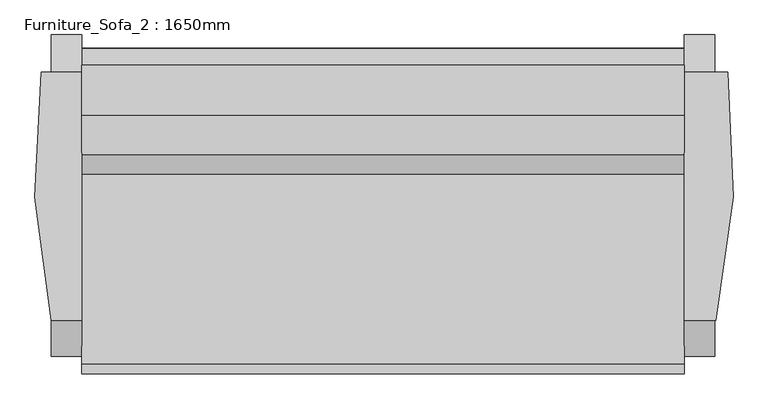
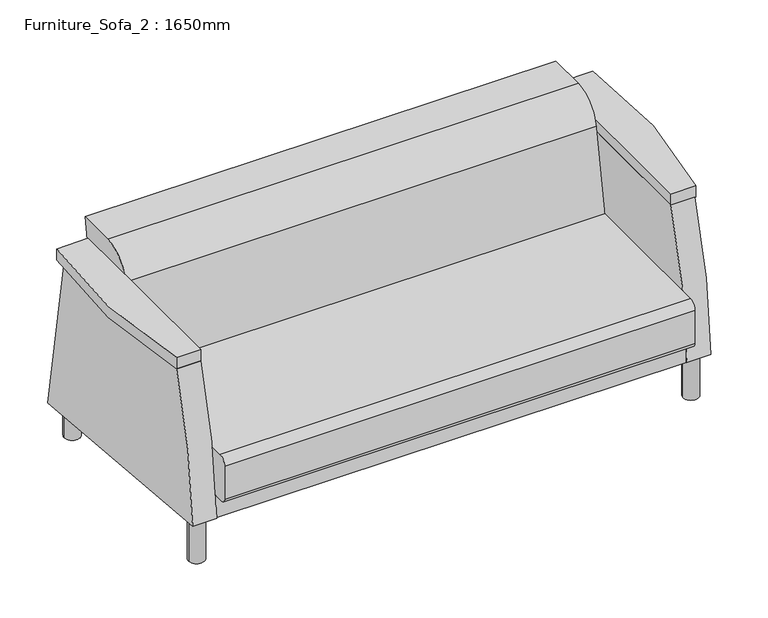
"""IFC4 building model written with IfcOpenShell, lengths in millimetres: furniture geometry, Furniture_Sofa_2 : 1650mm."""

from ifc_helpers import new_model, si_unit, point, frame, frame_2d, origin, origin_with_axes, place, context, project, spatial, polyline, circle_curve, trimmed, segment, composite_curve, outline, extrude, source, transform, mapped, element, save


def furniture_sofa_2_1650mm_c7211d0d(model_context):
    return source(origin(), model_context, "Body", "SweptSolid", [
        extrude(outline(composite_curve([segment(trimmed(circle_curve(frame_2d((-116.5901639, 351.2509954)), 25.4), [point((-141.9901639, 351.2509954))], [point((-116.5901639, 376.6509954))], False, "CARTESIAN"), True, "CONTINUOUS"), segment(polyline([(-116.5901639, 376.6509954), (355.3895541, 376.6509954), (402.1988177, 642.1195211)]), True, "CONTINUOUS"), segment(trimmed(circle_curve(frame_2d((502.2552854, 624.4768662)), 101.6), [point((402.1988177, 642.1195211))], [point((502.2552854, 726.0768662))], False, "CARTESIAN"), True, "CONTINUOUS"), segment(polyline([(502.2552854, 726.0768662), (626.3344485, 726.0768662), (609.5377828, 620.1719187), (667.6541767, 224.2509954), (-126.1151639, 224.2509954)]), True, "CONTINUOUS"), segment(trimmed(circle_curve(frame_2d((-126.1151639, 240.1259954)), 15.875), [point((-126.1151639, 224.2509954))], [point((-141.9901639, 240.1259954))], False, "CARTESIAN"), True, "CONTINUOUS"), segment(polyline([(-141.9901639, 240.1259954), (-141.9901639, 351.2509954)]), True, "CONTINUOUS")], self_intersect=False)), frame((-470.19375, 0.0, 0.0), z_axis=(1.0, 0.0, 0.0), x_axis=(0.0, 1.0, 0.0)), (0.0, 0.0, 1.0), 1497.6),
        extrude(outline(composite_curve([segment(polyline([(701.7619204, 79.3588346), (-97.7900405, 149.3105671)]), True, "CONTINUOUS"), segment(trimmed(circle_curve(frame_2d((1499.9783711, 99.5888442)), 1598.5418814), [point((-97.7900405, 149.3105671))], [point((-9.3943348, 626.0203985))], False, "CARTESIAN"), True, "CONTINUOUS"), segment(polyline([(-9.3943348, 626.0203985), (608.6917937, 626.0203985), (701.7619204, 79.3588346)]), True, "CONTINUOUS")], self_intersect=False)), frame((1027.40625, 0.0, 0.0), z_axis=(1.0, 0.0, 0.0), x_axis=(0.0, 1.0, 0.0)), (0.0, 0.0, 1.0), 76.2),
        extrude(outline(composite_curve([segment(polyline([(-9.3943348, 626.0203985), (608.6917937, 626.0203985), (701.7619204, 79.3588346), (-97.7900405, 149.3105671)]), True, "CONTINUOUS"), segment(trimmed(circle_curve(frame_2d((1499.9783711, 99.5888442)), 1598.5418814), [point((-97.7900405, 149.3105671))], [point((-9.3943348, 626.0203985))], False, "CARTESIAN"), True, "CONTINUOUS")], self_intersect=False)), frame((-546.39375, 0.0, 0.0), z_axis=(1.0, 0.0, 0.0), x_axis=(0.0, 1.0, 0.0)), (0.0, 0.0, 1.0), 76.2),
        extrude(outline(polyline([(1027.40625, 668.3047863), (1027.40625, -93.6952137), (-470.19375, -93.6952137), (-470.19375, 668.3047863), (1027.40625, 668.3047863)])), frame((0.0, 0.0, 148.0509954), z_axis=(0.0, 0.0, 1.0), x_axis=(1.0, 0.0, 0.0)), (0.0, 0.0, 1.0), 76.2),
        extrude(outline(composite_curve([segment(trimmed(circle_curve(frame_2d((-508.29375, -53.0901639)), 25.4), [point((-533.69375, -53.0901639))], [point((-482.89375, -53.0901639))], False, "CARTESIAN"), True, "CONTINUOUS"), segment(trimmed(circle_curve(frame_2d((-508.29375, -53.0901639)), 25.4), [point((-482.89375, -53.0901639))], [point((-533.69375, -53.0901639))], False, "CARTESIAN"), True, "CONTINUOUS")], self_intersect=False)), origin_with_axes(), (0.0, 0.0, 1.0), 148.43125),
        extrude(outline(composite_curve([segment(trimmed(circle_curve(frame_2d((-508.29375, 632.7098361)), 25.4), [point((-533.69375, 632.7098361))], [point((-482.89375, 632.7098361))], False, "CARTESIAN"), True, "CONTINUOUS"), segment(trimmed(circle_curve(frame_2d((-508.29375, 632.7098361)), 25.4), [point((-482.89375, 632.7098361))], [point((-533.69375, 632.7098361))], False, "CARTESIAN"), True, "CONTINUOUS")], self_intersect=False)), origin_with_axes(), (0.0, 0.0, 1.0), 148.43125),
        extrude(outline(composite_curve([segment(trimmed(circle_curve(frame_2d((1065.50625, 632.7098361)), 25.4), [point((1040.10625, 632.7098361))], [point((1090.90625, 632.7098361))], False, "CARTESIAN"), True, "CONTINUOUS"), segment(trimmed(circle_curve(frame_2d((1065.50625, 632.7098361)), 25.4), [point((1090.90625, 632.7098361))], [point((1040.10625, 632.7098361))], False, "CARTESIAN"), True, "CONTINUOUS")], self_intersect=False)), origin_with_axes(), (0.0, 0.0, 1.0), 148.43125),
        extrude(outline(composite_curve([segment(trimmed(circle_curve(frame_2d((1065.50625, -53.0901639)), 25.4), [point((1040.10625, -53.0901639))], [point((1090.90625, -53.0901639))], False, "CARTESIAN"), True, "CONTINUOUS"), segment(trimmed(circle_curve(frame_2d((1065.50625, -53.0901639)), 25.4), [point((1090.90625, -53.0901639))], [point((1040.10625, -53.0901639))], False, "CARTESIAN"), True, "CONTINUOUS")], self_intersect=False)), origin_with_axes(), (0.0, 0.0, 1.0), 148.43125),
        extrude(outline(composite_curve([segment(polyline([(-470.19375, -9.3943348), (-546.39375, -9.3943348)]), True, "CONTINUOUS"), segment(trimmed(circle_curve(frame_2d((1137.7527561, 369.3799517)), 1726.2153441), [point((-546.39375, -9.3943348))], [point((-571.79375, 608.6917935))], False, "CARTESIAN"), True, "CONTINUOUS"), segment(polyline([(-571.79375, 608.6917935), (-470.19375, 608.6917935), (-470.19375, -9.3943348)]), True, "CONTINUOUS")], self_intersect=False)), frame((0.0, 0.0, 626.0203985), z_axis=(0.0, 0.0, 1.0), x_axis=(1.0, 0.0, 0.0)), (0.0, 0.0, 1.0), 38.1),
        extrude(outline(composite_curve([segment(polyline([(1027.40625, -9.3943348), (1027.40625, 608.9395268), (1136.0864453, 608.9395268)]), True, "CONTINUOUS"), segment(trimmed(circle_curve(frame_2d((-579.5771494, 383.2634494)), 1730.4425047), [point((1136.0864453, 608.9395268))], [point((1105.7273117, -9.3943348))], False, "CARTESIAN"), True, "CONTINUOUS"), segment(polyline([(1105.7273117, -9.3943348), (1027.40625, -9.3943348)]), True, "CONTINUOUS")], self_intersect=False)), frame((0.0, 0.0, 626.0203985), z_axis=(0.0, 0.0, 1.0), x_axis=(1.0, 0.0, 0.0)), (0.0, 0.0, 1.0), 38.1),
    ])


if __name__ == "__main__":
    model = new_model("IFC4")
    model_context = context("Model", 3, world=origin())
    ifc_project = project(units=[si_unit("LENGTHUNIT", "METRE", prefix="MILLI")], contexts=[model_context])
    site = spatial("IfcSite", under=ifc_project)
    building = spatial("IfcBuilding", under=site)
    placement = place(None, origin())
    furniture_sofa_2_1650mm_shape = furniture_sofa_2_1650mm_c7211d0d(model_context)
    element("IfcFurniture", 1, ObjectType="Furniture_Sofa_2 : 1650mm", at=placement, inside=building, context=model_context, shape_type="MappedRepresentation", body=[
        mapped(furniture_sofa_2_1650mm_shape, transform((0.0, 0.0, 0.0), x_axis=(1.0, 0.0, 0.0), y_axis=(0.0, 1.0, 0.0), z_axis=(0.0, 0.0, 1.0))),
    ])
    save(model, "model.ifc")

# Revit data of these elements
# Type "Furniture_Sofa_2 : 1650mm"
#   Keynote = "N"
#   Length = 5' - 4.96063"
#   Material Sofa = Textile - Linen, Smooth
#   Material Frame = Metal - Chrome
#   Default Elevation = 0
# Element 1 (IfcFurniture, "Furniture_Sofa_2 : 1650mm")
#   Materials on its faces: "Textile - Linen, Smooth", "Metal - Chrome"
# Materials
#   "Textile - Linen, Smooth": class "Fabric", colour RGB 249 239 230, transparency 0
#   "Metal - Chrome": class "Metal", colour RGB 17 17 17, transparency 0
